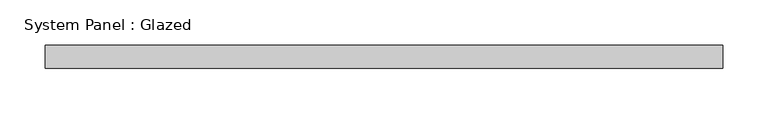
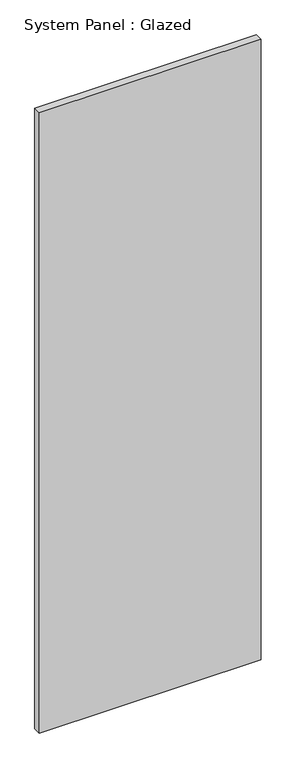
"""IFC4 building model written with IfcOpenShell, lengths in millimetres: plate geometry, System Panel : Glazed."""

from ifc_helpers import new_model, si_unit, origin, origin_with_axes, place, context, project, spatial, polyline, outline, extrude, source, transform, mapped, element, save


def system_panel_glazed_aa1e9ff3(model_context):
    return source(origin(), model_context, "Body", "SweptSolid", [
        extrude(outline(polyline([(373.9073867, 19.05), (-373.9073867, 19.05), (-373.9073867, 44.45), (373.9073867, 44.45), (373.9073867, 19.05)])), origin_with_axes(), (0.0, 0.0, 1.0), 2209.8),
    ])


if __name__ == "__main__":
    model = new_model("IFC4")
    model_context = context("Model", 3, world=origin())
    ifc_project = project(units=[si_unit("LENGTHUNIT", "METRE", prefix="MILLI")], contexts=[model_context])
    site = spatial("IfcSite", under=ifc_project)
    building = spatial("IfcBuilding", under=site)
    placement = place(None, origin())
    system_panel_glazed_shape = system_panel_glazed_aa1e9ff3(model_context)
    element("IfcPlate", 1, ObjectType="System Panel : Glazed", at=placement, inside=building, context=model_context, shape_type="MappedRepresentation", body=[
        mapped(system_panel_glazed_shape, transform((0.0, 0.0, 0.0), x_axis=(1.0, 0.0, 0.0), y_axis=(0.0, 1.0, 0.0), z_axis=(0.0, 0.0, 1.0))),
    ])
    save(model, "model.ifc")

# Revit data of these elements
# Type "System Panel : Glazed"
#   Construction Type Id = "GSP4R"
#   Analytic Construction = "1/8 in Pilkington single glazing"
#   Visual Light Transmittance = 0.9
#   Solar Heat Gain Coefficient = 0.86
#   Heat Transfer Coefficient (U) = 1.18115 BTU/(h·ft²·°F)
#   Define Thermal Properties by = 1
# Element 1 (IfcPlate, "System Panel : Glazed")
#   Materials on its faces: "Glass"
# Materials
#   "Glass": class "Glass", colour RGB 0 128 192, transparency 0.75, Description = "Soda Lime Glass", Cost = 0
